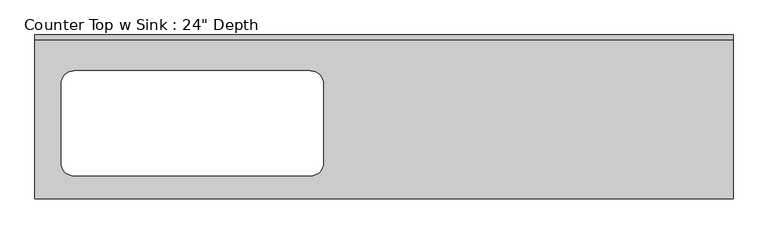
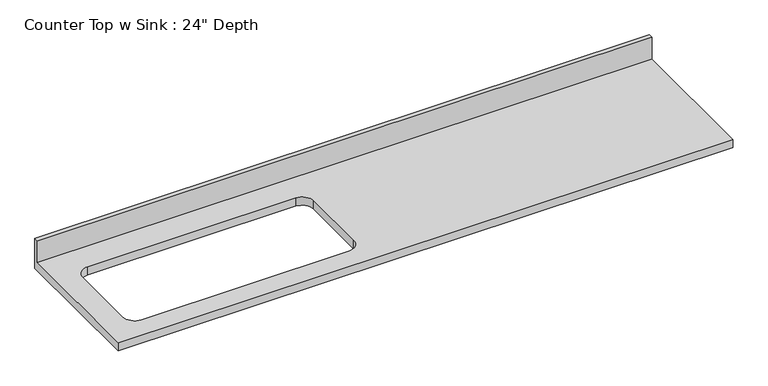
"""IFC4 building model written with IfcOpenShell, lengths in millimetres: furniture geometry."""

from ifc_helpers import new_model, si_unit, frame, origin, place, context, project, spatial, polyline, circle_curve, source, transform, mapped, element, save
from ifc_brep_helpers import plane_surface, revolved_surface, advanced_brep


def furniture_e2cf6ce7(model_context):
    return source(origin(), model_context, "Body", "AdvancedBrep", [
        advanced_brep(
        [(-1200.4622951, -635.0, 914.4), (1504.6377049, -635.0, 914.4), (1504.6377049, -19.05, 914.4), (-1200.4622951, -19.05, 914.4), (-1048.0622951, -139.7, 914.4), (-133.6622951, -139.7, 914.4), (-82.8622951, -190.5, 914.4), (-82.8622951, -495.3, 914.4), (-133.6622951, -546.1, 914.4), (-1048.0622951, -546.1, 914.4), (-1098.8622951, -495.3, 914.4), (-1098.8622951, -190.5, 914.4), (1504.6377049, 0.0, 876.3), (1504.6377049, -635.0, 876.3), (-1200.4622951, -635.0, 876.3), (-1200.4622951, 0.0, 876.3), (-133.6622951, -139.7, 876.3), (-1048.0622951, -139.7, 876.3), (-1098.8622951, -190.5, 876.3), (-1098.8622951, -495.3, 876.3), (-1048.0622951, -546.1, 876.3), (-133.6622951, -546.1, 876.3), (-82.8622951, -495.3, 876.3), (-82.8622951, -190.5, 876.3), (-1200.4622951, 0.0, 1016.0), (1504.6377049, 0.0, 1016.0), (-1200.4622951, -19.05, 1016.0), (1504.6377049, -19.05, 1016.0)],
        [
            (0, 1),
            (1, 2),
            (2, 3),
            (3, 0),
            (4, 5),
            (5, 6, circle_curve(frame((-133.6622951, -190.5, 914.4), z_axis=(0.0, 0.0, -1.0), x_axis=(1.0, 0.0, 0.0)), 50.8)),
            (6, 7),
            (7, 8, circle_curve(frame((-133.6622951, -495.3, 914.4), z_axis=(0.0, 0.0, -1.0), x_axis=(1.0, 0.0, 0.0)), 50.8)),
            (8, 9),
            (9, 10, circle_curve(frame((-1048.0622951, -495.3, 914.4), z_axis=(0.0, 0.0, -1.0), x_axis=(1.0, 0.0, 0.0)), 50.8)),
            (10, 11),
            (11, 4, circle_curve(frame((-1048.0622951, -190.5, 914.4), z_axis=(0.0, 0.0, -1.0), x_axis=(1.0, 0.0, 0.0)), 50.8)),
            (12, 13),
            (13, 14),
            (14, 15),
            (15, 12),
            (16, 17),
            (17, 18, circle_curve(frame((-1048.0622951, -190.5, 876.3), z_axis=(0.0, 0.0, 1.0), x_axis=(1.0, 0.0, 0.0)), 50.8)),
            (18, 19),
            (19, 20, circle_curve(frame((-1048.0622951, -495.3, 876.3), z_axis=(0.0, 0.0, 1.0), x_axis=(1.0, 0.0, 0.0)), 50.8)),
            (20, 21),
            (21, 22, circle_curve(frame((-133.6622951, -495.3, 876.3), z_axis=(0.0, 0.0, 1.0), x_axis=(1.0, 0.0, 0.0)), 50.8)),
            (22, 23),
            (23, 16, circle_curve(frame((-133.6622951, -190.5, 876.3), z_axis=(0.0, 0.0, 1.0), x_axis=(1.0, 0.0, 0.0)), 50.8)),
            (15, 24),
            (24, 25),
            (25, 12),
            (14, 0),
            (3, 26),
            (26, 24),
            (13, 1),
            (25, 27),
            (27, 2),
            (26, 27),
            (4, 17),
            (16, 5),
            (11, 18),
            (10, 19),
            (9, 20),
            (8, 21),
            (7, 22),
            (6, 23),
        ],
        [
            plane_surface(frame((-1200.4622951, 0.0, 914.4), z_axis=(0.0, 0.0, 1.0), x_axis=(-1.0, 0.0, 0.0))),
            plane_surface(frame((-1200.4622951, 0.0, 876.3), z_axis=(0.0, 0.0, -1.0), x_axis=(1.0, 0.0, 0.0))),
            plane_surface(frame((1504.6377049, 0.0, 914.4), z_axis=(0.0, 1.0, 0.0), x_axis=(0.0, 0.0, -1.0))),
            plane_surface(frame((-1200.4622951, 0.0, 914.4), z_axis=(-1.0, 0.0, 0.0), x_axis=(0.0, 0.0, -1.0))),
            plane_surface(frame((-1200.4622951, -635.0, 914.4), z_axis=(0.0, -1.0, 0.0), x_axis=(0.0, 0.0, -1.0))),
            plane_surface(frame((1504.6377049, -635.0, 914.4), z_axis=(1.0, 0.0, 0.0), x_axis=(0.0, 0.0, -1.0))),
            plane_surface(frame((-1200.4622951, 0.0, 1016.0), z_axis=(0.0, 0.0, 1.0), x_axis=(0.0, -1.0, 0.0))),
            plane_surface(frame((-1200.4622951, -19.05, 1016.0), z_axis=(0.0, -1.0, 0.0), x_axis=(0.0, 0.0, -1.0))),
            plane_surface(frame((-133.6622951, -139.7, 914.4), z_axis=(0.0, -1.0, 0.0), x_axis=(0.0, 0.0, -1.0))),
            revolved_surface(polyline([(-997.2622951000001, -190.5, 914.4), (-997.2622951000001, -190.5, 876.3)]), (-1048.0622951, -190.5, 876.3), (0.0, 0.0, 1.0)),
            plane_surface(frame((-1098.8622951, -190.5, 914.4), z_axis=(1.0, 0.0, 0.0), x_axis=(0.0, 0.0, -1.0))),
            revolved_surface(polyline([(-997.2622951000001, -495.3, 914.4), (-997.2622951000001, -495.3, 876.3)]), (-1048.0622951, -495.3, 876.3), (0.0, 0.0, 1.0)),
            plane_surface(frame((-1048.0622951, -546.1, 914.4), z_axis=(0.0, 1.0, 0.0), x_axis=(0.0, 0.0, -1.0))),
            revolved_surface(polyline([(-82.8622951, -495.3, 914.4), (-82.8622951, -495.3, 876.3)]), (-133.6622951, -495.3, 876.3), (0.0, 0.0, 1.0)),
            plane_surface(frame((-82.8622951, -495.3, 914.4), z_axis=(-1.0, 0.0, 0.0), x_axis=(0.0, 0.0, -1.0))),
            revolved_surface(polyline([(-82.8622951, -190.5, 914.4), (-82.8622951, -190.5, 876.3)]), (-133.6622951, -190.5, 876.3), (0.0, 0.0, 1.0)),
        ],
        [
            (0, [[1, 2, 3, 4], [5, 6, 7, 8, 9, 10, 11, 12]]),
            (1, [[13, 14, 15, 16], [17, 18, 19, 20, 21, 22, 23, 24]]),
            (2, [[-16, 25, 26, 27]]),
            (3, [[-15, 28, -4, 29, 30, -25]]),
            (4, [[-1, -28, -14, 31]]),
            (5, [[-13, -27, 32, 33, -2, -31]]),
            (6, [[-30, 34, -32, -26]]),
            (7, [[-34, -29, -3, -33]]),
            (8, [[35, -17, 36, -5]]),
            (9, [[-35, -12, 37, -18]]),
            (10, [[-37, -11, 38, -19]]),
            (11, [[-38, -10, 39, -20]]),
            (12, [[-39, -9, 40, -21]]),
            (13, [[-40, -8, 41, -22]]),
            (14, [[-41, -7, 42, -23]]),
            (15, [[-36, -24, -42, -6]]),
        ],
    ),
    ])


if __name__ == "__main__":
    model = new_model("IFC4")
    model_context = context("Model", 3, world=origin())
    ifc_project = project(units=[si_unit("LENGTHUNIT", "METRE", prefix="MILLI")], contexts=[model_context])
    site = spatial("IfcSite", under=ifc_project)
    building = spatial("IfcBuilding", under=site)
    placement = place(None, origin())
    furniture_shape = furniture_e2cf6ce7(model_context)
    element("IfcFurniture", 1, ObjectType="Counter Top w Sink : 24\" Depth", at=placement, inside=building, context=model_context, shape_type="MappedRepresentation", body=[
        mapped(furniture_shape, transform((0.0, 0.0, 0.0), x_axis=(1.0, 0.0, 0.0), y_axis=(0.0, 1.0, 0.0), z_axis=(0.0, 0.0, 1.0))),
    ])
    save(model, "model.ifc")

# Revit data of these elements
# Type "Counter Top w Sink : 24\" Depth"
#   Assembly Code = "C1030400"
#   Counter Thickness = 0' - 1 1/2"
#   Depth = 2' - 1"
#   Height = 3' - 0"
#   Length [instance default] = 8' - 0"
#   Sink Location [instance default] = 2' - 0"
#   Sink Location To Wall [instance default] = 0' - 6"
#   Sink Opening Depth [instance default] = 1' - 3"
#   Sink Opening Width [instance default] = 3' - 3"
#   Counter Top Material = none
#   Default Elevation = 0
# Element 1 (IfcFurniture, "Counter Top w Sink : 24\" Depth")
#   Length = 8' - 10 1/2"
#   Materials on its faces: "Counter Top"
# Materials
#   "Counter Top": class "Wood", colour RGB 226 177 128, transparency 0
